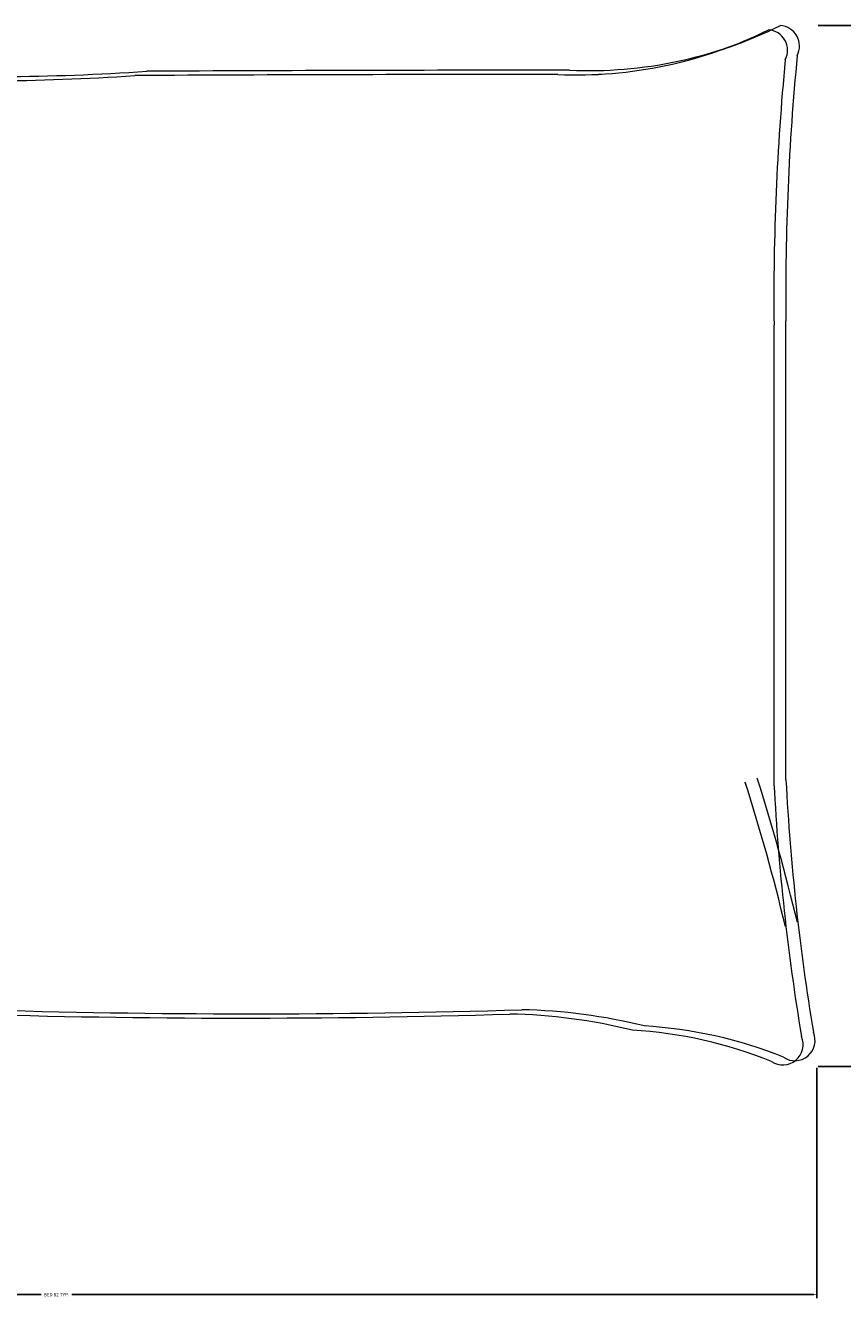
# Model space of a CAD drawing. Units: inches. Extents: x 2168 to 3056, y 1130 to 2629.
# Tile 28 of 42: x 2505 to 2549, y 2307 to 2376. Entities that reach past the tile are written whole.
import ezdxf

# ---------------------------------------------------------------- set-up
doc = ezdxf.new("R2010")
doc.units = ezdxf.units.IN
doc.layers.add('A-ANNO-DIMS', color=2, linetype='Continuous', lineweight=18)
doc.layers.add('A-FURN', color=8, linetype='Continuous', lineweight=13)
doc.styles.get("Standard").update_dxf_attribs({"font": 'arial.ttf'})
doc.dimstyles.get("Standard").update_dxf_attribs({"dimtxt": 0.18, "dimasz": 0.18, "dimexe": 0.18, "dimexo": 0.0625, "dimgap": 0.09, "dimtad": 0, "dimtih": 1, "dimtoh": 1, "dimdec": 4, "dimzin": 0, "dimdsep": 46, "dimtxsty": 'Standard', "dimcen": 0.09, "dimadec": 0, "dimazin": 0, "dimtfac": 1, "dimtdec": 4, "dimtofl": 0, "dimtmove": 0, "dimatfit": 3, "dimfxl": 1, "dimtolj": 1, "dimtzin": 0, "dimarcsym": 0})

# ---------------------------------------------------------------- blocks, each defined once
blk = doc.blocks.new('BED-DOUBLE')
for p, q in [((79.885, 15.292), (79.885, 39.906)), ((79.885, 15.292), (79.885, 39.905)), ((79.245, 15.064), (79.245, 39.677)), ((79.245, 15.063), (79.245, 39.677))]:
    blk.add_line(p, q)
for centre, radius, start, end in [((68.667, 76.158), 23.065, 267.47136, 296.46809), ((68.667, 76.157), 23.065, 267.47136, 296.46809), ((69.306, 76.386), 23.065, 267.47136, 296.46809), ((69.306, 76.386), 23.065, 267.47136, 296.46809), ((78.87, 54.41), 1.102, 332.65876, 86.02002), ((78.87, 54.41), 1.102, 332.65876, 86.02002), ((79.51, 54.639), 1.102, 332.65876, 86.02002), ((79.51, 54.638), 1.102, 332.65876, 86.02002), ((212.916, 41.38), 133.04, 174.4998, 180.63509), ((212.916, 41.38), 133.04, 174.4998, 180.63509), ((212.277, 41.152), 133.04, 174.4998, 180.63509), ((212.277, 41.152), 133.04, 174.4998, 180.63509), ((36.315, 182.266), 129.499, 266.97912, 273.83645), ((36.315, 182.266), 129.499, 266.97912, 273.83645), ((36.955, 182.494), 129.499, 266.97912, 273.83645), ((36.955, 182.494), 129.499, 266.97912, 273.83645), ((67.822, -4508.743), 4561.858, 90.002168, 90.286887), ((67.822, -4508.744), 4561.858, 90.002168, 90.286887), ((68.461, -4508.515), 4561.858, 90.002168, 90.286887), ((68.461, -4508.515), 4561.858, 90.002168, 90.286887), ((-23.712, -17.221), 106.459, 13.38322, 17.70533), ((-23.712, -17.222), 106.459, 13.38322, 17.70533), ((-23.072, -16.993), 106.459, 13.38322, 17.70533), ((-23.072, -16.993), 106.459, 13.38322, 17.70533), ((201.477, 21.655), 121.759, 182.99578, 189.40907), ((201.477, 21.655), 121.759, 182.99578, 189.40907), ((200.837, 21.427), 121.759, 182.99578, 189.40907), ((200.837, 21.427), 121.759, 182.99578, 189.40907), ((50.614, 484.823), 482.31, 268.22771, 271.71854), ((50.614, 484.822), 482.31, 268.22771, 271.71854), ((51.253, 485.051), 482.31, 268.22771, 271.71854), ((51.253, 485.051), 482.31, 268.22771, 271.71854), ((65.155, -26.671), 29.634, 76.06484, 88.91125), ((65.155, -26.671), 29.634, 76.06484, 88.91125), ((64.515, -26.899), 29.634, 76.06484, 88.91125), ((64.515, -26.9), 29.634, 76.06484, 88.91125), ((70.915, -21.431), 23.562, 67.97508, 86.652), ((70.915, -21.431), 23.562, 67.97508, 86.652), ((70.276, -21.659), 23.562, 67.97508, 86.652), ((70.276, -21.66), 23.562, 67.97508, 86.652), ((79.718, 1.088), 1.089, 236.17358, 23.47814), ((79.718, 1.087), 1.089, 236.17358, 23.47814), ((80.357, 1.316), 1.089, 236.17358, 23.47814), ((80.357, 1.316), 1.089, 236.17358, 23.47814)]:
    blk.add_arc(centre, radius, start, end)
blk = doc.blocks.new('*D14')
at = {"layer": 'A-ANNO-DIMS', "color": 0, "lineweight": -2, "transparency": 16777216}
for p, q in [((2466.224, 2319.873), (2466.224, 2307.523)), ((2547.772, 2319.873), (2547.772, 2307.523)), ((2466.404, 2307.703), (2506.18, 2307.703)), ((2547.592, 2307.703), (2507.815, 2307.703))]:
    blk.add_line(p, q, dxfattribs=at)
at = {"layer": 'A-ANNO-DIMS', "color": 0, "transparency": 16777216}
for points in [[(2466.404, 2307.733), (2466.404, 2307.673), (2466.224, 2307.703)], [(2547.592, 2307.733), (2547.592, 2307.673), (2547.772, 2307.703)]]:
    blk.add_solid(points, dxfattribs=at)
at = {"layer": 'Defpoints', "color": 0, "transparency": 16777216}
for p in [(2466.224, 2319.935), (2547.772, 2319.935), (2547.772, 2307.703)]:
    blk.add_point(p, dxfattribs=at)
at = {"layer": 'A-ANNO-DIMS', "color": 0, "transparency": 16777216, "insert": (2506.998, 2307.703), "char_height": 0.18, "attachment_point": 5}
blk.add_mtext('\\A1;BED 82 TYP.', dxfattribs=at)
blk = doc.blocks.new('*D15')
at = {"layer": 'A-ANNO-DIMS', "color": 0, "lineweight": -2, "transparency": 16777216}
for p, q in [((2547.835, 2375.76), (2560.185, 2375.76)), ((2560.005, 2375.58), (2560.005, 2348.029)), ((2560.005, 2320.115), (2560.005, 2347.665)), ((2547.835, 2319.935), (2560.185, 2319.935))]:
    blk.add_line(p, q, dxfattribs=at)
at = {"layer": 'A-ANNO-DIMS', "color": 0, "transparency": 16777216}
for points in [[(2559.975, 2375.58), (2560.035, 2375.58), (2560.005, 2375.76)], [(2559.975, 2320.115), (2560.035, 2320.115), (2560.005, 2319.935)]]:
    blk.add_solid(points, dxfattribs=at)
at = {"layer": 'Defpoints', "color": 0, "transparency": 16777216}
for p in [(2547.772, 2375.76), (2560.005, 2375.76), (2547.772, 2319.935)]:
    blk.add_point(p, dxfattribs=at)
at = {"layer": 'A-ANNO-DIMS', "color": 0, "transparency": 16777216, "insert": (2560.005, 2347.847), "char_height": 0.18, "attachment_point": 5}
blk.add_mtext('\\A1;56 TYP.', dxfattribs=at)

msp = doc.modelspace()

# ---------------------------------------------------------------- block references
at = {"layer": 'A-FURN'}
msp.add_blockref('BED-DOUBLE', (2466.223, 2320.021), dxfattribs=at)

# ---------------------------------------------------------------- dimensions: what is measured, and where the dimension line sits
at = {"layer": 'A-ANNO-DIMS'}
dim = msp.add_linear_dim(base=(2560.005, 2375.76), p1=(2547.772, 2319.935), p2=(2547.772, 2375.76), angle=90, text='<> TYP.', dimstyle='Standard', override={"dimdec": 0, "dimlfac": 1, "dimrnd": 0, "dimzin": 0, "dimdsep": 46, "dimlunit": 2}, dxfattribs=at)
dim.commit()
dim.dimension.update_dxf_attribs({"geometry": '*D15', "text_midpoint": (2560.005, 2347.847)})
dim = msp.add_linear_dim(base=(2547.772, 2307.703), p1=(2466.224, 2319.935), p2=(2547.772, 2319.935), text='BED <> TYP.', dimstyle='Standard', override={"dimdec": 0, "dimlfac": 1, "dimrnd": 0, "dimzin": 0, "dimdsep": 46, "dimlunit": 2}, dxfattribs=at)
dim.commit()
dim.dimension.update_dxf_attribs({"geometry": '*D14', "text_midpoint": (2506.998, 2307.703)})

doc.saveas('drawing.dxf')
